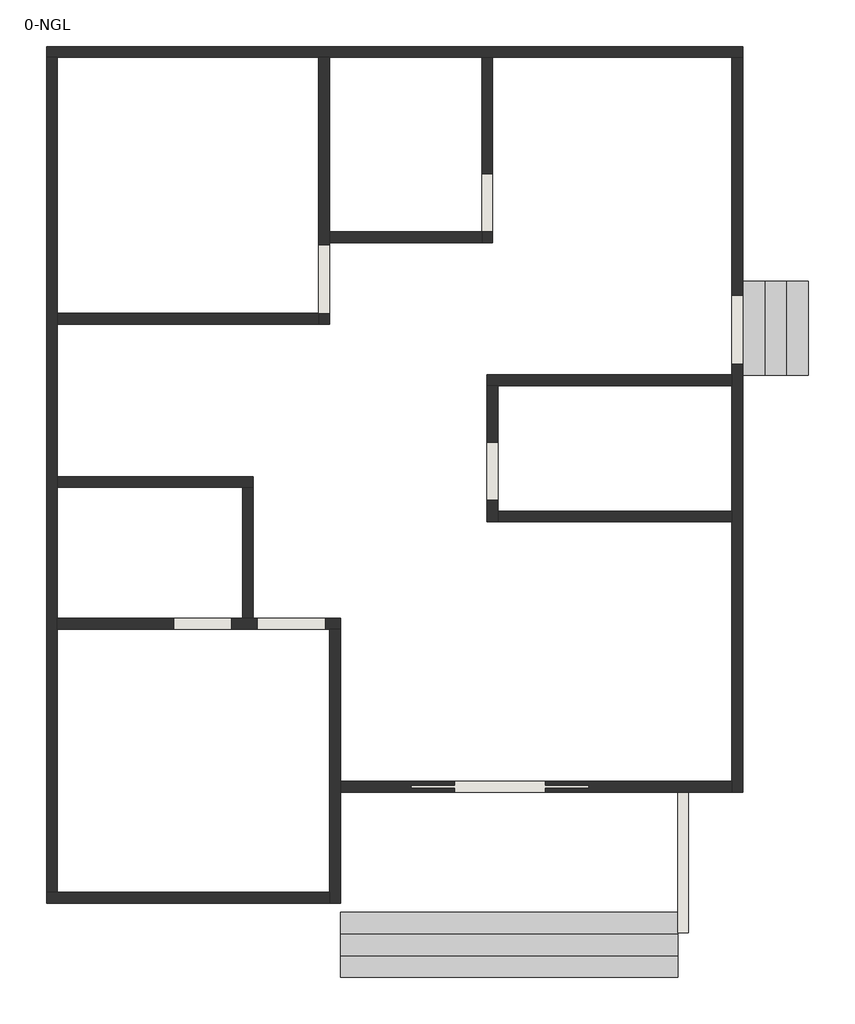
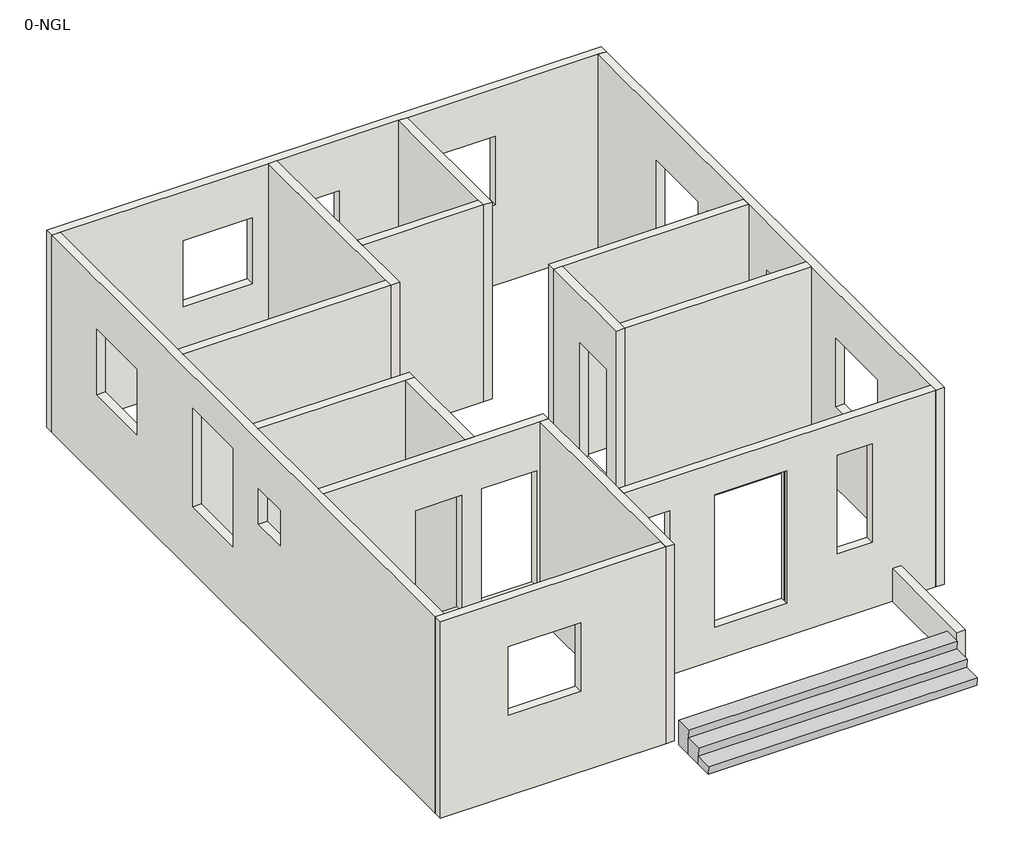
# One storey: 17 walls, 2 stair flights.
"""IFC4 building model written with IfcOpenShell, lengths in millimetres."""

from ifc_helpers import new_model, si_unit, origin, origin_with_axes, place, context, project, spatial, polyline, outline, extrude, faceted_brep, element, save

model = new_model("IFC4")

# Units and contexts
model_context = context("Model", 3, world=origin())
ifc_project = project(units=[si_unit("LENGTHUNIT", "METRE", prefix="MILLI")], contexts=[model_context])

# Site, building, storey
site = spatial("IfcSite", under=ifc_project)
building = spatial("IfcBuilding", under=site)
storey = spatial("IfcBuildingStorey", under=building, Name="0-NGL", Elevation=0.0)

# Stair flights
placement = place(None, origin())
element("IfcStairFlight", 1, ObjectType="00-stairs", at=placement, inside=storey, context=model_context, shape_type="Brep", body=[
    faceted_brep([(2945.3465688, -1632.4647803, 152.4), (-1779.0534312, -1632.4647803, 152.4), (-1779.0534312, -1613.4147803, 0.0), (2945.3465688, -1613.4147803, 0.0), (2945.3465688, -1308.6147803, 152.4), (-1779.0534312, -1308.6147803, 152.4), (-1779.0534312, -1308.6147803, 0.0), (2945.3465688, -1308.6147803, 0.0), (-1779.0534312, -1327.6647803, 304.8), (2945.3465688, -1327.6647803, 304.8), (2945.3465688, -1003.8147803, 304.8), (-1779.0534312, -1003.8147803, 304.8), (-1779.0534312, -1003.8147803, 0.0), (2945.3465688, -1003.8147803, 0.0), (-1779.0534312, -1022.8647803, 457.2), (2945.3465688, -1022.8647803, 457.2), (2945.3465688, -718.0647803, 457.2), (-1779.0534312, -718.0647803, 457.2), (-1779.0534312, -718.0647803, 0.0), (2945.3465688, -718.0647803, 0.0)], [[[0, 1, 2, 3]], [[1, 0, 4, 5]], [[1, 5, 6, 2]], [[4, 0, 3, 7]], [[8, 9, 10, 11]], [[6, 5, 8, 11, 12]], [[4, 7, 13, 10, 9]], [[5, 4, 9, 8]], [[14, 15, 16, 17]], [[12, 11, 14, 17, 18]], [[10, 13, 19, 16, 15]], [[17, 16, 19, 18]], [[11, 10, 15, 14]], [[2, 6, 12, 18, 19, 13, 7, 3]]]),
])
element("IfcStairFlight", 2, ObjectType="00-stairs", at=placement, inside=storey, context=model_context, shape_type="Brep", body=[
    faceted_brep([(4774.1465688, 8115.7655428, 152.4), (4774.1465688, 6794.9655428, 152.4), (4755.0965688, 6794.9655428, 0.0), (4755.0965688, 8115.7655428, 0.0), (4450.2965688, 8115.7655428, 152.4), (4450.2965688, 6794.9655428, 152.4), (4450.2965688, 6794.9655428, 0.0), (4450.2965688, 8115.7655428, 0.0), (4469.3465688, 6794.9655428, 304.8), (4469.3465688, 8115.7655428, 304.8), (4145.4965688, 8115.7655428, 304.8), (4145.4965688, 6794.9655428, 304.8), (4145.4965688, 6794.9655428, 0.0), (4145.4965688, 8115.7655428, 0.0), (4164.5465688, 6794.9655428, 457.2), (4164.5465688, 8115.7655428, 457.2), (3859.7465688, 8115.7655428, 457.2), (3859.7465688, 6794.9655428, 457.2), (3859.7465688, 6794.9655428, 0.0), (3859.7465688, 8115.7655428, 0.0)], [[[0, 1, 2, 3]], [[1, 0, 4, 5]], [[1, 5, 6, 2]], [[4, 0, 3, 7]], [[8, 9, 10, 11]], [[6, 5, 8, 11, 12]], [[4, 7, 13, 10, 9]], [[5, 4, 9, 8]], [[14, 15, 16, 17]], [[12, 11, 14, 17, 18]], [[10, 13, 19, 16, 15]], [[17, 16, 19, 18]], [[11, 10, 15, 14]], [[2, 6, 12, 18, 19, 13, 7, 3]]]),
])

# Walls
element("IfcWall", 3, ObjectType="6\" INNER WALL", at=placement, inside=storey, context=model_context, shape_type="Brep", body=[
    faceted_brep([(-5893.8534312, 11245.3352197, 0.0), (-5741.4534312, 11245.3352197, 0.0), (-2083.8534312, 11245.3352197, 0.0), (-1931.4534312, 11245.3352197, 0.0), (202.1465688, 11245.3352197, 0.0), (354.5465688, 11245.3352197, 0.0), (3707.3465688, 11245.3352197, 0.0), (3859.7465688, 11245.3352197, 0.0), (3859.7465688, 11245.3352197, 3657.6), (3707.3465688, 11245.3352197, 3657.6), (354.5465688, 11245.3352197, 3657.6), (202.1465688, 11245.3352197, 3657.6), (-1931.4534312, 11245.3352197, 3657.6), (-2083.8534312, 11245.3352197, 3657.6), (-5741.4534312, 11245.3352197, 3657.6), (-5893.8534312, 11245.3352197, 3657.6), (-2363.2534312, 11245.3352197, 2743.2), (-2363.2534312, 11245.3352197, 1524.0), (-3582.4534312, 11245.3352197, 1524.0), (-3582.4534312, 11245.3352197, 2743.2), (-839.6534312, 11245.3352197, 1753.8), (-1499.2534312, 11245.3352197, 1753.8), (-1499.2534312, 11245.3352197, 2718.2), (-839.6534312, 11245.3352197, 2718.2), (1903.5465688, 11245.3352197, 1499.0), (634.3465688, 11245.3352197, 1499.0), (634.3465688, 11245.3352197, 2768.2), (1903.5465688, 11245.3352197, 2768.2), (3859.7465688, 11397.7352197, 0.0), (-5893.8534312, 11397.7352197, 0.0), (-5893.8534312, 11397.7352197, 3657.6), (3859.7465688, 11397.7352197, 3657.6), (-2363.2534312, 11397.7352197, 1524.0), (-2363.2534312, 11397.7352197, 2743.2), (-3582.4534312, 11397.7352197, 2743.2), (-3582.4534312, 11397.7352197, 1524.0), (-839.6534312, 11397.7352197, 1753.8), (-839.6534312, 11397.7352197, 2718.2), (-1499.2534312, 11397.7352197, 2718.2), (-1499.2534312, 11397.7352197, 1753.8), (1903.5465688, 11397.7352197, 1499.0), (1903.5465688, 11397.7352197, 2768.2), (634.3465688, 11397.7352197, 2768.2), (634.3465688, 11397.7352197, 1499.0)], [[[0, 1, 2, 3, 4, 5, 6, 7, 8, 9, 10, 11, 12, 13, 14, 15], [16, 17, 18, 19], [20, 21, 22, 23], [24, 25, 26, 27]], [[28, 29, 30, 31], [32, 33, 34, 35], [36, 37, 38, 39], [40, 41, 42, 43]], [[7, 6, 5, 4, 3, 2, 1, 0, 29, 28]], [[15, 14, 13, 12, 11, 10, 9, 8, 31, 30]], [[8, 7, 28, 31]], [[0, 15, 30, 29]], [[32, 17, 16, 33]], [[33, 16, 19, 34]], [[34, 19, 18, 35]], [[17, 32, 35, 18]], [[37, 36, 20, 23]], [[38, 37, 23, 22]], [[39, 38, 22, 21]], [[36, 39, 21, 20]], [[41, 40, 24, 27]], [[42, 41, 27, 26]], [[43, 42, 26, 25]], [[40, 43, 25, 24]]]),
])
element("IfcWall", 4, ObjectType="6\" INNER WALL", at=placement, inside=storey, context=model_context, shape_type="Brep", body=[
    faceted_brep([(3707.3465688, 11245.3352197, 0.0), (3707.3465688, 6800.3352197, 0.0), (3707.3465688, 6647.9352197, 0.0), (3707.3465688, 4895.3352197, 0.0), (3707.3465688, 4742.9352197, 0.0), (3707.3465688, 1110.7352197, 0.0), (3707.3465688, 958.3352197, 0.0), (3707.3465688, 958.3352197, 3657.6), (3707.3465688, 1110.7352197, 3657.6), (3707.3465688, 4742.9352197, 3657.6), (3707.3465688, 4895.3352197, 3657.6), (3707.3465688, 6647.9352197, 3657.6), (3707.3465688, 6800.3352197, 3657.6), (3707.3465688, 11245.3352197, 3657.6), (3707.3465688, 6952.7352197, 2768.6), (3707.3465688, 6952.7352197, 609.6), (3707.3465688, 7917.9352197, 609.6), (3707.3465688, 7917.9352197, 2768.6), (3707.3465688, 5441.8352197, 2768.2), (3707.3465688, 5441.8352197, 2108.6), (3707.3465688, 6101.4352197, 2108.6), (3707.3465688, 6101.4352197, 2768.2), (3707.3465688, 8197.7352197, 2768.2), (3707.3465688, 8197.7352197, 1499.0), (3707.3465688, 9466.9352197, 1499.0), (3707.3465688, 9466.9352197, 2768.2), (3707.3465688, 4005.9352197, 1499.0), (3707.3465688, 4005.9352197, 2768.2), (3707.3465688, 2736.7352197, 2768.2), (3707.3465688, 2736.7352197, 1499.0), (3859.7465688, 958.3352197, 0.0), (3859.7465688, 11245.3352197, 0.0), (3859.7465688, 11245.3352197, 3657.6), (3859.7465688, 958.3352197, 3657.6), (3859.7465688, 6952.7352197, 609.6), (3859.7465688, 6952.7352197, 2768.6), (3859.7465688, 7917.9352197, 2768.6), (3859.7465688, 7917.9352197, 609.6), (3859.7465688, 5441.8352197, 2108.6), (3859.7465688, 5441.8352197, 2768.2), (3859.7465688, 6101.4352197, 2768.2), (3859.7465688, 6101.4352197, 2108.6), (3859.7465688, 8197.7352197, 1499.0), (3859.7465688, 8197.7352197, 2768.2), (3859.7465688, 9466.9352197, 2768.2), (3859.7465688, 9466.9352197, 1499.0), (3859.7465688, 4005.9352197, 1499.0), (3859.7465688, 2736.7352197, 1499.0), (3859.7465688, 2736.7352197, 2768.2), (3859.7465688, 4005.9352197, 2768.2)], [[[0, 1, 2, 3, 4, 5, 6, 7, 8, 9, 10, 11, 12, 13], [14, 15, 16, 17], [18, 19, 20, 21], [22, 23, 24, 25], [26, 27, 28, 29]], [[30, 31, 32, 33], [34, 35, 36, 37], [38, 39, 40, 41], [42, 43, 44, 45], [46, 47, 48, 49]], [[6, 5, 4, 3, 2, 1, 0, 31, 30]], [[13, 12, 11, 10, 9, 8, 7, 33, 32]], [[0, 13, 32, 31]], [[7, 6, 30, 33]], [[35, 34, 15, 14]], [[36, 35, 14, 17]], [[37, 36, 17, 16]], [[34, 37, 16, 15]], [[39, 38, 19, 18]], [[40, 39, 18, 21]], [[41, 40, 21, 20]], [[38, 41, 20, 19]], [[43, 42, 23, 22]], [[44, 43, 22, 25]], [[45, 44, 25, 24]], [[42, 45, 24, 23]], [[27, 26, 46, 49]], [[28, 27, 49, 48]], [[29, 28, 48, 47]], [[26, 29, 47, 46]]]),
])
element("IfcWall", 5, ObjectType="6\" INNER WALL", at=placement, inside=storey, context=model_context, shape_type="Brep", body=[
    faceted_brep([(3707.3465688, 1110.7352197, 0.0), (-1779.0534312, 1110.7352197, 0.0), (-1779.0534312, 1110.7352197, 3657.6), (3707.3465688, 1110.7352197, 3657.6), (1091.1465688, 1110.7352197, 3073.4), (-178.8534312, 1110.7352197, 3073.4), (-178.8534312, 1110.7352197, 609.6), (1091.1465688, 1110.7352197, 609.6), (1980.1465688, 1110.7352197, 3048.0), (1980.1465688, 1110.7352197, 1219.2), (2589.7465688, 1110.7352197, 1219.2), (2589.7465688, 1110.7352197, 3048.0), (-1575.8534312, 1110.7352197, 3048.0), (-1575.8534312, 1110.7352197, 1219.2), (-966.2534312, 1110.7352197, 1219.2), (-966.2534312, 1110.7352197, 3048.0), (-1779.0534312, 958.3352197, 0.0), (2945.3465688, 958.3352197, 0.0), (3097.7465688, 958.3352197, 0.0), (3707.3465688, 958.3352197, 0.0), (3707.3465688, 958.3352197, 3657.6), (-1779.0534312, 958.3352197, 3657.6), (-178.8534312, 958.3352197, 3073.4), (1091.1465688, 958.3352197, 3073.4), (1091.1465688, 958.3352197, 609.6), (-178.8534312, 958.3352197, 609.6), (1980.1465688, 958.3352197, 1219.2), (1980.1465688, 958.3352197, 3048.0), (2589.7465688, 958.3352197, 3048.0), (2589.7465688, 958.3352197, 1219.2), (-1575.8534312, 958.3352197, 1219.2), (-1575.8534312, 958.3352197, 3048.0), (-966.2534312, 958.3352197, 3048.0), (-966.2534312, 958.3352197, 1219.2), (-788.4534312, 1013.8977197, 3073.4), (-788.4534312, 1055.1727197, 3073.4), (-178.8534312, 1055.1727197, 3073.4), (1091.1465688, 1055.1727197, 3073.4), (1700.7465688, 1055.1727197, 3073.4), (1700.7465688, 1013.8977197, 3073.4), (1091.1465688, 1013.8977197, 3073.4), (-178.8534312, 1013.8977197, 3073.4), (-788.4534312, 1013.8977197, 609.6), (-178.8534312, 1013.8977197, 609.6), (1091.1465688, 1013.8977197, 609.6), (1700.7465688, 1013.8977197, 609.6), (1700.7465688, 1055.1727197, 609.6), (1091.1465688, 1055.1727197, 609.6), (-178.8534312, 1055.1727197, 609.6), (-788.4534312, 1055.1727197, 609.6)], [[[0, 1, 2, 3], [4, 5, 6, 7], [8, 9, 10, 11], [12, 13, 14, 15]], [[16, 17, 18, 19, 20, 21], [22, 23, 24, 25], [26, 27, 28, 29], [30, 31, 32, 33]], [[1, 0, 19, 18, 17, 16]], [[3, 2, 21, 20]], [[0, 3, 20, 19]], [[2, 1, 16, 21]], [[34, 35, 36, 5, 4, 37, 38, 39, 40, 23, 22, 41]], [[42, 43, 25, 24, 44, 45, 46, 47, 7, 6, 48, 49]], [[34, 41, 43, 42]], [[41, 22, 25, 43]], [[23, 40, 44, 24]], [[40, 39, 45, 44]], [[39, 38, 46, 45]], [[38, 37, 47, 46]], [[37, 4, 7, 47]], [[5, 36, 48, 6]], [[36, 35, 49, 48]], [[35, 34, 42, 49]], [[8, 27, 26, 9]], [[27, 8, 11, 28]], [[28, 11, 10, 29]], [[9, 26, 29, 10]], [[30, 13, 12, 31]], [[31, 12, 15, 32]], [[32, 15, 14, 33]], [[13, 30, 33, 14]]]),
])
element("IfcWall", 6, ObjectType="6\" INNER WALL", at=placement, inside=storey, context=model_context, shape_type="SweptSolid", body=[
    extrude(outline(polyline([(-3150.6534312, 3396.7352197), (-3150.6534312, 5225.5352197), (-2998.2534312, 5225.5352197), (-2998.2534312, 3396.7352197), (-3150.6534312, 3396.7352197)])), origin_with_axes(), (0.0, 0.0, 1.0), 3657.6),
])
element("IfcWall", 7, ObjectType="6\" INNER WALL", at=placement, inside=storey, context=model_context, shape_type="Brep", body=[
    faceted_brep([(-5741.4534312, -438.6647803, 0.0), (-5741.4534312, 3244.3352197, 0.0), (-5741.4534312, 3396.7352197, 0.0), (-5741.4534312, 5225.5352197, 0.0), (-5741.4534312, 5377.9352197, 0.0), (-5741.4534312, 7511.5352197, 0.0), (-5741.4534312, 7663.9352197, 0.0), (-5741.4534312, 11245.3352197, 0.0), (-5741.4534312, 11245.3352197, 3657.6), (-5741.4534312, 7663.9352197, 3657.6), (-5741.4534312, 7511.5352197, 3657.6), (-5741.4534312, 5377.9352197, 3657.6), (-5741.4534312, 5225.5352197, 3657.6), (-5741.4534312, 3396.7352197, 3657.6), (-5741.4534312, 3244.3352197, 3657.6), (-5741.4534312, -438.6647803, 3657.6), (-5741.4534312, 6946.3852197, 3048.0), (-5741.4534312, 6946.3852197, 1219.2), (-5741.4534312, 5727.1852197, 1219.2), (-5741.4534312, 5727.1852197, 3048.0), (-5741.4534312, 9873.7352197, 2743.2), (-5741.4534312, 9873.7352197, 1524.0), (-5741.4534312, 8654.5352197, 1524.0), (-5741.4534312, 8654.5352197, 2743.2), (-5741.4534312, 4286.1352197, 2108.6), (-5741.4534312, 4286.1352197, 2768.2), (-5741.4534312, 4945.7352197, 2768.2), (-5741.4534312, 4945.7352197, 2108.6), (-5893.8534312, 11245.3352197, 0.0), (-5893.8534312, -438.6647803, 0.0), (-5893.8534312, -438.6647803, 3657.6), (-5893.8534312, 11245.3352197, 3657.6), (-5893.8534312, 6946.3852197, 1219.2), (-5893.8534312, 6946.3852197, 3048.0), (-5893.8534312, 5727.1852197, 3048.0), (-5893.8534312, 5727.1852197, 1219.2), (-5893.8534312, 9873.7352197, 1524.0), (-5893.8534312, 9873.7352197, 2743.2), (-5893.8534312, 8654.5352197, 2743.2), (-5893.8534312, 8654.5352197, 1524.0), (-5893.8534312, 4286.1352197, 2768.2), (-5893.8534312, 4286.1352197, 2108.6), (-5893.8534312, 4945.7352197, 2108.6), (-5893.8534312, 4945.7352197, 2768.2)], [[[0, 1, 2, 3, 4, 5, 6, 7, 8, 9, 10, 11, 12, 13, 14, 15], [16, 17, 18, 19], [20, 21, 22, 23], [24, 25, 26, 27]], [[28, 29, 30, 31], [32, 33, 34, 35], [36, 37, 38, 39], [40, 41, 42, 43]], [[7, 6, 5, 4, 3, 2, 1, 0, 29, 28]], [[15, 14, 13, 12, 11, 10, 9, 8, 31, 30]], [[8, 7, 28, 31]], [[0, 15, 30, 29]], [[32, 17, 16, 33]], [[33, 16, 19, 34]], [[34, 19, 18, 35]], [[17, 32, 35, 18]], [[20, 37, 36, 21]], [[37, 20, 23, 38]], [[38, 23, 22, 39]], [[21, 36, 39, 22]], [[25, 24, 41, 40]], [[26, 25, 40, 43]], [[27, 26, 43, 42]], [[24, 27, 42, 41]]]),
])
element("IfcWall", 8, ObjectType="6\" INNER WALL", at=placement, inside=storey, context=model_context, shape_type="Brep", body=[
    faceted_brep([(-2083.8534312, 11245.3352197, 0.0), (-2083.8534312, 7663.9352197, 0.0), (-2083.8534312, 7511.5352197, 0.0), (-2083.8534312, 7511.5352197, 3657.6), (-2083.8534312, 7663.9352197, 3657.6), (-2083.8534312, 11245.3352197, 3657.6), (-2083.8534312, 7658.386397, 609.6), (-2083.8534312, 8623.586397, 609.6), (-2083.8534312, 8623.586397, 2768.6), (-2083.8534312, 7658.386397, 2768.6), (-1931.4534312, 11245.3352197, 0.0), (-1931.4534312, 11245.3352197, 3657.6), (-1931.4534312, 8806.9352197, 3657.6), (-1931.4534312, 8654.5352197, 3657.6), (-1931.4534312, 7511.5352197, 3657.6), (-1931.4534312, 7511.5352197, 0.0), (-1931.4534312, 8654.5352197, 0.0), (-1931.4534312, 8806.9352197, 0.0), (-1931.4534312, 7658.386397, 609.6), (-1931.4534312, 7658.386397, 2768.6), (-1931.4534312, 8623.586397, 2768.6), (-1931.4534312, 8623.586397, 609.6)], [[[0, 1, 2, 3, 4, 5], [6, 7, 8, 9]], [[10, 11, 12, 13, 14, 15, 16, 17], [18, 19, 20, 21]], [[2, 1, 0, 10, 17, 16, 15]], [[5, 4, 3, 14, 13, 12, 11]], [[0, 5, 11, 10]], [[3, 2, 15, 14]], [[19, 18, 6, 9]], [[20, 19, 9, 8]], [[21, 20, 8, 7]], [[18, 21, 7, 6]]]),
])
element("IfcWall", 9, ObjectType="6\" INNER WALL", at=placement, inside=storey, context=model_context, shape_type="SweptSolid", body=[
    extrude(outline(polyline([(-5741.4534312, 7663.9352197), (-2083.8534312, 7663.9352197), (-2083.8534312, 7511.5352197), (-5741.4534312, 7511.5352197), (-5741.4534312, 7663.9352197)])), origin_with_axes(), (0.0, 0.0, 1.0), 3657.6),
])
element("IfcWall", 10, ObjectType="6\" INNER WALL", at=placement, inside=storey, context=model_context, shape_type="Brep", body=[
    faceted_brep([(202.1465688, 11245.3352197, 0.0), (202.1465688, 8806.9352197, 0.0), (202.1465688, 8654.5352197, 0.0), (202.1465688, 8654.5352197, 3657.6), (202.1465688, 8806.9352197, 3657.6), (202.1465688, 11245.3352197, 3657.6), (202.1465688, 8806.9352197, 609.6), (202.1465688, 9619.7352197, 609.6), (202.1465688, 9619.7352197, 2768.6), (202.1465688, 8806.9352197, 2768.6), (354.5465688, 11245.3352197, 0.0), (354.5465688, 11245.3352197, 3657.6), (354.5465688, 8654.5352197, 3657.6), (354.5465688, 8654.5352197, 0.0), (354.5465688, 8806.9352197, 609.6), (354.5465688, 8806.9352197, 2768.6), (354.5465688, 9619.7352197, 2768.6), (354.5465688, 9619.7352197, 609.6)], [[[0, 1, 2, 3, 4, 5], [6, 7, 8, 9]], [[10, 11, 12, 13], [14, 15, 16, 17]], [[2, 1, 0, 10, 13]], [[5, 4, 3, 12, 11]], [[0, 5, 11, 10]], [[3, 2, 13, 12]], [[15, 14, 6, 9]], [[16, 15, 9, 8]], [[17, 16, 8, 7]], [[14, 17, 7, 6]]]),
])
element("IfcWall", 11, ObjectType="6\" INNER WALL", at=placement, inside=storey, context=model_context, shape_type="SweptSolid", body=[
    extrude(outline(polyline([(-1931.4534312, 8806.9352197), (202.1465688, 8806.9352197), (202.1465688, 8654.5352197), (-1931.4534312, 8654.5352197), (-1931.4534312, 8806.9352197)])), origin_with_axes(), (0.0, 0.0, 1.0), 3657.6),
])
element("IfcWall", 12, ObjectType="6\" INNER WALL", at=placement, inside=storey, context=model_context, shape_type="Brep", body=[
    faceted_brep([(-5741.4534312, 5225.5352197, 0.0), (-3150.6534312, 5225.5352197, 0.0), (-2998.2534312, 5225.5352197, 0.0), (-2998.2534312, 5225.5352197, 3657.6), (-3150.6534312, 5225.5352197, 3657.6), (-5741.4534312, 5225.5352197, 3657.6), (-5741.4534312, 5377.9352197, 0.0), (-5741.4534312, 5377.9352197, 3657.6), (-2998.2534312, 5377.9352197, 3657.6), (-2998.2534312, 5377.9352197, 0.0)], [[[0, 1, 2, 3, 4, 5]], [[6, 7, 8, 9]], [[2, 1, 0, 6, 9]], [[5, 4, 3, 8, 7]], [[0, 5, 7, 6]], [[3, 2, 9, 8]]]),
])
element("IfcWall", 13, ObjectType="6\" INNER WALL", at=placement, inside=storey, context=model_context, shape_type="Brep", body=[
    faceted_brep([(-1779.0534312, 3396.7352197, 0.0), (-2998.2534312, 3396.7352197, 0.0), (-3150.6534312, 3396.7352197, 0.0), (-5741.4534312, 3396.7352197, 0.0), (-5741.4534312, 3396.7352197, 3657.6), (-3150.6534312, 3396.7352197, 3657.6), (-2998.2534312, 3396.7352197, 3657.6), (-1779.0534312, 3396.7352197, 3657.6), (-1982.2534312, 3396.7352197, 609.6), (-1982.2534312, 3396.7352197, 2768.6), (-2947.4534312, 3396.7352197, 2768.6), (-2947.4534312, 3396.7352197, 609.6), (-3303.0534312, 3396.7352197, 609.6), (-3303.0534312, 3396.7352197, 2768.6), (-4115.8534312, 3396.7352197, 2768.6), (-4115.8534312, 3396.7352197, 609.6), (-1779.0534312, 3244.3352197, 0.0), (-1779.0534312, 3244.3352197, 3657.6), (-1931.4534312, 3244.3352197, 3657.6), (-5741.4534312, 3244.3352197, 3657.6), (-5741.4534312, 3244.3352197, 0.0), (-1931.4534312, 3244.3352197, 0.0), (-1982.2534312, 3244.3352197, 609.6), (-2947.4534312, 3244.3352197, 609.6), (-2947.4534312, 3244.3352197, 2768.6), (-1982.2534312, 3244.3352197, 2768.6), (-3303.0534312, 3244.3352197, 609.6), (-4115.8534312, 3244.3352197, 609.6), (-4115.8534312, 3244.3352197, 2768.6), (-3303.0534312, 3244.3352197, 2768.6)], [[[0, 1, 2, 3, 4, 5, 6, 7], [8, 9, 10, 11], [12, 13, 14, 15]], [[16, 17, 18, 19, 20, 21], [22, 23, 24, 25], [26, 27, 28, 29]], [[3, 2, 1, 0, 16, 21, 20]], [[7, 6, 5, 4, 19, 18, 17]], [[4, 3, 20, 19]], [[0, 7, 17, 16]], [[9, 8, 22, 25]], [[10, 9, 25, 24]], [[11, 10, 24, 23]], [[8, 11, 23, 22]], [[13, 12, 26, 29]], [[14, 13, 29, 28]], [[15, 14, 28, 27]], [[12, 15, 27, 26]]]),
])
element("IfcWall", 14, ObjectType="6\" INNER WALL", at=placement, inside=storey, context=model_context, shape_type="Brep", body=[
    faceted_brep([(3707.3465688, 6800.3352197, 0.0), (278.3465688, 6800.3352197, 0.0), (278.3465688, 6800.3352197, 3657.6), (3707.3465688, 6800.3352197, 3657.6), (3707.3465688, 6647.9352197, 0.0), (3707.3465688, 6647.9352197, 3657.6), (430.7465688, 6647.9352197, 3657.6), (278.3465688, 6647.9352197, 3657.6), (278.3465688, 6647.9352197, 0.0), (430.7465688, 6647.9352197, 0.0)], [[[0, 1, 2, 3]], [[4, 5, 6, 7, 8, 9]], [[1, 0, 4, 9, 8]], [[3, 2, 7, 6, 5]], [[0, 3, 5, 4]], [[2, 1, 8, 7]]]),
])
element("IfcWall", 15, ObjectType="6\" INNER WALL", at=placement, inside=storey, context=model_context, shape_type="Brep", body=[
    faceted_brep([(278.3465688, 6647.9352197, 0.0), (278.3465688, 4742.9352197, 0.0), (278.3465688, 4742.9352197, 3657.6), (278.3465688, 6647.9352197, 3657.6), (278.3465688, 5047.7352197, 609.6), (278.3465688, 5860.5352197, 609.6), (278.3465688, 5860.5352197, 2768.6), (278.3465688, 5047.7352197, 2768.6), (430.7465688, 6647.9352197, 0.0), (430.7465688, 6647.9352197, 3657.6), (430.7465688, 4895.3352197, 3657.6), (430.7465688, 4742.9352197, 3657.6), (430.7465688, 4742.9352197, 0.0), (430.7465688, 4895.3352197, 0.0), (430.7465688, 5047.7352197, 609.6), (430.7465688, 5047.7352197, 2768.6), (430.7465688, 5860.5352197, 2768.6), (430.7465688, 5860.5352197, 609.6)], [[[0, 1, 2, 3], [4, 5, 6, 7]], [[8, 9, 10, 11, 12, 13], [14, 15, 16, 17]], [[1, 0, 8, 13, 12]], [[3, 2, 11, 10, 9]], [[0, 3, 9, 8]], [[2, 1, 12, 11]], [[15, 14, 4, 7]], [[16, 15, 7, 6]], [[17, 16, 6, 5]], [[14, 17, 5, 4]]]),
])
element("IfcWall", 16, ObjectType="6\" INNER WALL", at=placement, inside=storey, context=model_context, shape_type="SweptSolid", body=[
    extrude(outline(polyline([(3707.3465688, 4742.9352197), (430.7465688, 4742.9352197), (430.7465688, 4895.3352197), (3707.3465688, 4895.3352197), (3707.3465688, 4742.9352197)])), origin_with_axes(), (0.0, 0.0, 1.0), 3657.6),
])
element("IfcWall", 17, ObjectType="6\" INNER WALL", at=placement, inside=storey, context=model_context, shape_type="Brep", body=[
    faceted_brep([(-1931.4534312, 3244.3352197, 0.0), (-1931.4534312, -438.6647803, 0.0), (-1931.4534312, -591.0647803, 0.0), (-1931.4534312, -591.0647803, 3657.6), (-1931.4534312, -438.6647803, 3657.6), (-1931.4534312, 3244.3352197, 3657.6), (-1779.0534312, 3244.3352197, 0.0), (-1779.0534312, 3244.3352197, 3657.6), (-1779.0534312, 1110.7352197, 3657.6), (-1779.0534312, 958.3352197, 3657.6), (-1779.0534312, -591.0647803, 3657.6), (-1779.0534312, -591.0647803, 0.0), (-1779.0534312, 958.3352197, 0.0), (-1779.0534312, 1110.7352197, 0.0)], [[[0, 1, 2, 3, 4, 5]], [[6, 7, 8, 9, 10, 11, 12, 13]], [[2, 1, 0, 6, 13, 12, 11]], [[5, 4, 3, 10, 9, 8, 7]], [[0, 5, 7, 6]], [[3, 2, 11, 10]]]),
])
element("IfcWall", 18, ObjectType="6\" INNER WALL", at=placement, inside=storey, context=model_context, shape_type="Brep", body=[
    faceted_brep([(-1931.4534312, -438.6647803, 0.0), (-5741.4534312, -438.6647803, 0.0), (-5893.8534312, -438.6647803, 0.0), (-5893.8534312, -438.6647803, 3657.6), (-5741.4534312, -438.6647803, 3657.6), (-1931.4534312, -438.6647803, 3657.6), (-4699.6534312, -438.6647803, 1499.0), (-3430.4534312, -438.6647803, 1499.0), (-3430.4534312, -438.6647803, 2768.2), (-4699.6534312, -438.6647803, 2768.2), (-1931.4534312, -591.0647803, 0.0), (-1931.4534312, -591.0647803, 3657.6), (-5893.8534312, -591.0647803, 3657.6), (-5893.8534312, -591.0647803, 0.0), (-4699.6534312, -591.0647803, 1499.0), (-4699.6534312, -591.0647803, 2768.2), (-3430.4534312, -591.0647803, 2768.2), (-3430.4534312, -591.0647803, 1499.0)], [[[0, 1, 2, 3, 4, 5], [6, 7, 8, 9]], [[10, 11, 12, 13], [14, 15, 16, 17]], [[2, 1, 0, 10, 13]], [[5, 4, 3, 12, 11]], [[3, 2, 13, 12]], [[15, 14, 6, 9]], [[16, 15, 9, 8]], [[17, 16, 8, 7]], [[14, 17, 7, 6]], [[0, 5, 11, 10]]]),
])
element("IfcWall", 19, ObjectType="6\" INNER WALL", at=placement, inside=storey, context=model_context, shape_type="SweptSolid", body=[
    extrude(outline(polyline([(2945.3465688, -1003.8147803), (2945.3465688, 958.3352197), (3097.7465688, 958.3352197), (3097.7465688, -1003.8147803), (2945.3465688, -1003.8147803)])), origin_with_axes(), (0.0, 0.0, 1.0), 609.6),
])

save(model, "model.ifc")

# Revit data of these elements
# Type "6\" INNER WALL"
#   Assembly Code = "B2010"
#   Layers, outside or top first: 0' - 6" "00-9\" MAIN WALL" (function 1)
# Elements 1, 2 (IfcStairFlight, "00-stairs")
#   Phase Created = New Construction
#   Materials on its faces: "Concrete, Cast-in-Place gray"
# Elements 3, 4, 5, 6, 7, 8, 9, 10, 11, 12, 13, 14, 15, 16, 17, 18 (IfcWall, "6\" INNER WALL")
#   Top Offset = 0' - 0"
#   Base Offset = 0' - 0"
#   wall height = 12' - 0"
#   Phase Created = New Construction
#   Base Constraint = 0-NGL
#   Top Constraint = 2-FIRST FLOOR
#   Materials on its faces: "00-9\" MAIN WALL"
# Element 19 (IfcWall, "6\" INNER WALL")
#   Top Offset = 0' - 0"
#   Base Offset = 0' - 0"
#   wall height = 2' - 0"
#   Phase Created = New Construction
#   Base Constraint = 0-NGL
#   Top Constraint = 1-PL
#   Materials on its faces: "00-9\" MAIN WALL"
# Materials
#   "00-9\" MAIN WALL": class "Generic", colour RGB 244 244 244, transparency 0, Cost = 0
#   "Concrete, Cast-in-Place gray": class "Concrete", colour RGB 192 192 192, transparency 0, Description = "Cast-in-place concrete", Cost = 0
